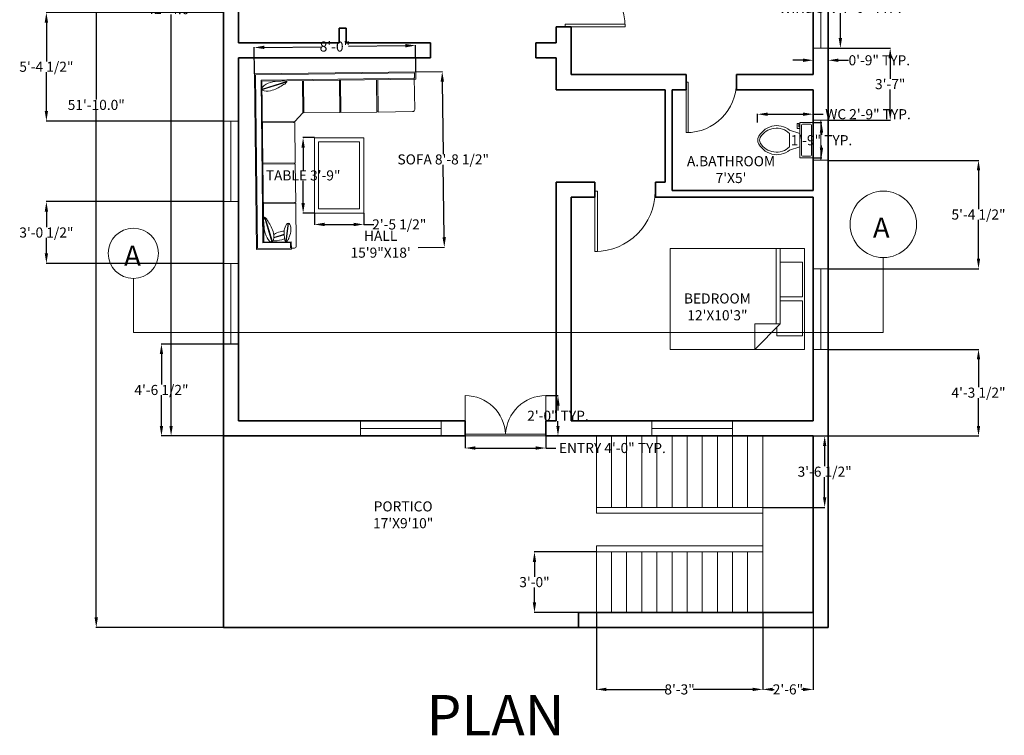
# Model space of a CAD drawing. Units: inches. Extents: x 94 to 277359, y -289541 to 1081.
# Tile 2 of 5: x 94 to 680, y 339 to 765. Entities that reach past the tile are written whole.
import ezdxf

# ---------------------------------------------------------------- set-up
doc = ezdxf.new("R2010")
doc.units = ezdxf.units.IN
doc.header["$MEASUREMENT"] = 0
doc.layers.get('Defpoints').update_dxf_attribs({"color": 255})
for name, color, linetype, lineweight in [('A-ANNO-DIMS', 2, 'Continuous', 18), ('A-ANNO-SYMB', 7, 'Continuous', 18), ('A-ANNO-TEXT', 7, 'Continuous', 30), ('A-AREA-IDEN', 7, 'Continuous', 18), ('A-DOOR', 4, 'Continuous', 18), ('A-FLOR-FIXT', 8, 'Continuous', 18), ('A-WALL', 7, 'Continuous', 35), ('furniture', 163, 'Continuous', 18), ('STAIRCASE', 10, 'Continuous', 18), ('window', 13, 'Continuous', 18)]:
    doc.layers.add(name, color=color, linetype=linetype, lineweight=lineweight)
doc.styles.get("Standard").update_dxf_attribs({"font": 'arial.ttf'})
doc.dimstyles.get("Standard").update_dxf_attribs({"dimtxt": 6, "dimasz": 6, "dimexe": 0.18, "dimexo": 0.0625, "dimgap": 0.09, "dimtad": 0, "dimtih": 1, "dimtoh": 1, "dimdec": 1, "dimzin": 0, "dimdsep": 46, "dimlunit": 3, "dimtxsty": 'Standard', "dimcen": 0.09, "dimadec": 0, "dimazin": 0, "dimtfac": 1, "dimtdec": 1, "dimtofl": 0, "dimtmove": 0, "dimatfit": 3, "dimfxl": 1, "dimtolj": 1, "dimtzin": 0, "dimarcsym": 0})

# ---------------------------------------------------------------- blocks, each defined once
blk = doc.blocks.new('DOOR')
for p, q in [((-94.95, 365.26), (-85.95, 365.26)), ((-94.95, 317.26), (-94.95, 365.26)), ((-90.45, 365.26), (-90.45, 317.26)), ((-85.95, 365.26), (-85.95, 317.26)), ((-85.95, 317.26), (-94.95, 317.26))]:
    blk.add_line(p, q)
blk = doc.blocks.new('V')
for p, q in [((-17.52, 401.92), (-8.52, 401.92)), ((-17.52, 377.92), (-17.52, 401.92)), ((-13.02, 377.92), (-13.02, 401.92)), ((-8.52, 401.92), (-8.52, 377.92)), ((-8.52, 377.92), (-17.52, 377.92))]:
    blk.add_line(p, q)
blk = doc.blocks.new('*D3')
at = {"layer": 'A-ANNO-DIMS', "color": 0, "lineweight": -2, "transparency": 16777216}
for p, q in [((215.5, 1025.45), (139.73, 1025.45)), ((139.91, 1019.45), (139.91, 717.61)), ((139.91, 409.45), (139.91, 711.3)), ((215.5, 403.45), (139.73, 403.45))]:
    blk.add_line(p, q, dxfattribs=at)
at = {"layer": 'A-ANNO-DIMS', "color": 0, "transparency": 16777216}
for points in [[(138.91, 1019.45), (140.91, 1019.45), (139.91, 1025.45)], [(138.91, 409.45), (140.91, 409.45), (139.91, 403.45)]]:
    blk.add_solid(points, dxfattribs=at)
at = {"layer": 'Defpoints', "color": 0, "transparency": 16777216}
for p in [(139.91, 1025.45), (215.56, 1025.45), (215.56, 403.45)]:
    blk.add_point(p, dxfattribs=at)
at = {"layer": 'A-ANNO-DIMS', "color": 0, "transparency": 16777216, "insert": (139.91, 714.45), "char_height": 6, "attachment_point": 5}
blk.add_mtext('\\A1;51\'-10.0"', dxfattribs=at)
blk = doc.blocks.new('*D4')
at = {"layer": 'A-ANNO-DIMS', "color": 0, "lineweight": -2, "transparency": 16777216}
for p, q in [((215.5, 1025.45), (184.27, 1025.45)), ((184.45, 1019.45), (184.45, 774.61)), ((184.45, 523.45), (184.45, 768.3)), ((215.5, 517.45), (184.27, 517.45))]:
    blk.add_line(p, q, dxfattribs=at)
at = {"layer": 'A-ANNO-DIMS', "color": 0, "transparency": 16777216}
for points in [[(183.45, 1019.45), (185.45, 1019.45), (184.45, 1025.45)], [(183.45, 523.45), (185.45, 523.45), (184.45, 517.45)]]:
    blk.add_solid(points, dxfattribs=at)
at = {"layer": 'Defpoints', "color": 0, "transparency": 16777216}
for p in [(215.56, 1025.45), (184.45, 517.45), (215.56, 517.45)]:
    blk.add_point(p, dxfattribs=at)
at = {"layer": 'A-ANNO-DIMS', "color": 0, "transparency": 16777216, "insert": (184.45, 771.45), "char_height": 6, "attachment_point": 5}
blk.add_mtext('\\A1;42\'-4.0"', dxfattribs=at)
blk = doc.blocks.new('sofa')
at = {"layer": 'furniture'}
for p, q in [((350.79, 469.57), (336.2, 465.25)), ((350.63, 469.16), (336.28, 464.99)), ((383.04, 450.77), (383.04, 470.07)), ((406.99, 470.07), (406.99, 450.77)), ((430.99, 455.52), (426.82, 469.87)), ((431.39, 455.35), (427.08, 469.94)), ((338.43, 464.07), (340.23, 457.88)), ((338.72, 464.05), (340.51, 457.89)), ((332.19, 451.9), (332.19, 453.72)), ((336.18, 456.71), (347.07, 455.29)), ((336.2, 456.92), (347.1, 455.5)), ((359.61, 451.29), (358.97, 451.29)), ((359.61, 451.29), (358.97, 451.29)), ((383.04, 451.29), (382.4, 451.29)), ((407.63, 451.29), (406.99, 451.29)), ((358.97, 450.77), (333.46, 450.77)), ((382.39, 450.77), (359.61, 450.77)), ((406.99, 450.77), (383.04, 450.77)), ((413.11, 445.31), (413.11, 445.95)), ((413.11, 423.23), (413.11, 423.87)), ((413.11, 401.16), (413.11, 401.8)), ((413.87, 379.35), (432.81, 379.35))]:
    blk.add_line(p, q, dxfattribs=at)
for points in [[(431.89, 470.07), (431.89, 378.38), (436.22, 378.38), (436.22, 474.39), (331.68, 474.39), (331.68, 453.72), (336.08, 453.73), (336.08, 470.07), (431.89, 470.07)], [(358.97, 450.77), (358.97, 470.07)], [(359.61, 450.77), (359.61, 470.07)], [(382.4, 450.77), (382.4, 470.07)], [(431.89, 445.95), (412.6, 445.95), (407.63, 450.77), (407.63, 470.07)], [(431.89, 423.87), (412.6, 423.87), (412.6, 445.31), (431.89, 445.31)], [(412.6, 401.8), (412.6, 423.23), (431.89, 423.23)], [(431.89, 401.8), (412.6, 401.8)], [(412.6, 380.48), (412.6, 401.16), (431.89, 401.16)]]:
    blk.add_lwpolyline(points, dxfattribs=at)
blk.add_lwpolyline([(335.57, 470.58), (432.4, 470.58), (432.4, 379.24), (435.71, 379.24), (435.71, 473.88), (332.19, 473.88), (332.19, 454.23), (335.57, 454.23)], close=True, dxfattribs=at)
for centre, start, end in [((333.46, 452.05), 186.69307, 269.99993), ((413.87, 380.63), 180.00473, 270.00007)]:
    blk.add_arc(centre, 1.28, start, end, dxfattribs=at)
for points, knots in [([(349.6, 468.13), (349.14, 467.92), (347.75, 466.93), (344.77, 465.38), (341.49, 463.98), (336.52, 463.91), (335.8, 466.54), (340.37, 469.29), (344.16, 469.84), (347.43, 469.89), (349.25, 470.15), (351.26, 469.6), (349.6, 468.13)], [0, 0, 0, 0, 5.78506, 20.019226, 35.456927, 51.784724, 57.97649, 75.904696, 98.086664, 106.437957, 110.953168, 112.080004, 112.080004, 112.080004, 112.080004]), ([(429.95, 456.54), (429.75, 457.01), (428.75, 458.4), (427.21, 461.38), (425.8, 464.66), (425.74, 469.63), (428.37, 470.34), (431.12, 465.78), (431.67, 461.98), (431.72, 458.71), (431.98, 456.9), (431.42, 454.88), (429.95, 456.54)], [0, 0, 0, 0, 5.78506, 20.019226, 35.456927, 51.784724, 57.97649, 75.904696, 98.086664, 106.437957, 110.953168, 112.080004, 112.080004, 112.080004, 112.080004]), ([(337.88, 457.68), (337.9, 457.81), (337.02, 459.85), (336.72, 461.9), (336.65, 464.24), (336.65, 464.58)], [75.416636, 75.416636, 75.416636, 75.416636, 75.904696, 98.086664, 101.64289, 101.64289, 101.64289, 101.64289]), ([(340.47, 464.13), (340.65, 463.77), (341.43, 462.19), (342.13, 460.56), (342.38, 458.63), (342.46, 457.86)], [127.65261, 127.65261, 127.65261, 127.65261, 132.09923, 147.536931, 150.407473, 150.407473, 150.407473, 150.407473]), ([(336.4, 457.25), (336.73, 457.47), (338.07, 457.76), (340.75, 457.94), (343.6, 457.92), (347.27, 456.37), (346.95, 454.21), (342.72, 453.66), (339.77, 454.47), (337.35, 455.49), (336.22, 456.2), (336.14, 456.75), (336.4, 457.25)], [0, 0, 0, 0, 5.78506, 20.019226, 35.456927, 51.784724, 57.97649, 75.904696, 98.086664, 106.437957, 110.953168, 112.080004, 112.080004, 112.080004, 112.080004])]:
    blk.add_open_spline(points, degree=3, knots=knots, dxfattribs=at)
blk = doc.blocks.new('Bed - Queen')
for p, q in [((0, -80.00003), (0, 0)), ((0, 0), (59.99999, 0)), ((59.99999, 0), (59.99999, -80.00003)), ((7.99999, -1.2), (28.79998, -1.2)), ((7.99999, -14.4), (7.99999, -1.2)), ((28.79998, -1.2), (28.79998, -14.4)), ((31.19999, -1.2), (51.99999, -1.2)), ((31.19999, -14.4), (31.19999, -1.2)), ((51.99999, -1.2), (51.99999, -16.4)), ((0, -14.4), (44.8, -14.4)), ((44.8, -16.8), (0, -16.8)), ((59.99999, -29.6), (44.8, -14.4)), ((44.8, -14.4), (44.8, -29.6)), ((51.99999, -16.4), (46.79936, -16.4)), ((44.8, -29.6), (59.99999, -29.6)), ((59.99999, -80.00003), (0, -80.00003))]:
    blk.add_line(p, q)
blk = doc.blocks.new('taBLE')
at = {"layer": 'furniture'}
for points in [[(384.8, 484.44), (429.71, 484.44), (429.71, 455.08), (384.8, 455.08)], [(387.27, 481.97), (427.24, 481.97), (427.24, 457.55), (387.27, 457.55)]]:
    blk.add_lwpolyline(points, close=True, dxfattribs=at)
blk = doc.blocks.new('Toilet - top')
for p, q in [((9.5, -6), (9.5, -2)), ((-10, -8.5), (-8, -8.5)), ((-10, -9.5), (-10, -8.5)), ((-7, -9.5), (-10, -9.5)), ((-8, -8.5), (-8, -8)), ((-7, -8), (-7, -9.5)), ((-4, -8), (-6, -14)), ((4, -8), (6, -14)), ((4, -14), (-4, -14))]:
    blk.add_line(p, q)
blk.add_lwpolyline([(10.5, -8), (10.5, 0), (-10.5, 0), (-10.5, -8)], close=True)
for points in [[(-9.5, -2), (-9.5, -6)], [(8.5, -1), (-8.5, -1)], [(-8.5, -7), (8.5, -7)]]:
    blk.add_lwpolyline(points)
for centre, radius, start, end in [((-8.62, -1.88), 0.884, 81.8699, 188.1301), ((8.62, -1.88), 0.884, 351.8699, 98.1301), ((-8.62, -6.12), 0.884, 171.8699, 278.1301), ((8.62, -6.12), 0.884, 261.8699, 8.1301), ((3.52, -21.58), 12.17, 141.46911, 247.97143), ((4.2, -21.82), 11.33, 136.36773, 238.94682), ((-3.52, -21.58), 12.17, 292.02843, 38.53071), ((-4.2, -21.82), 11.33, 301.05301, 43.63209), ((0, -27.88), 4, 245.73182, 294.26817), ((0, -29), 4, 254.86053, 285.13947)]:
    blk.add_arc(centre, radius, start, end)
blk = doc.blocks.new('MD')
for p, q in [((202.8, 674.18), (202.8, 698.18)), ((250.8, 674.18), (250.8, 698.18)), ((202.8, 675.18), (250.8, 675.18)), ((202.8, 674.18), (250.8, 674.18))]:
    blk.add_line(p, q)
for centre, start, end in [((202.8, 674.18), 2.38802, 90), ((250.8, 674.18), 90, 177.61198)]:
    blk.add_arc(centre, 24, start, end)
blk = doc.blocks.new('*U15')
for p, q in [((0, 0), (0, -6)), ((40, 0), (40, -6))]:
    blk.add_line(p, q)
blk.add_lwpolyline([(0, 0), (0, 40), (1.75, 40), (1.75, 0)], close=True)
blk.add_arc((0, 0), 40, 0, 90)
blk = doc.blocks.new('*D21')
at = {"layer": 'A-ANNO-DIMS', "color": 0, "lineweight": -2, "transparency": 16777216}
for p, q in [((575.63, 796.21), (582.94, 796.21)), ((582.76, 790.21), (582.76, 775.41)), ((582.76, 754.21), (582.76, 769.02)), ((575.63, 748.21), (582.94, 748.21))]:
    blk.add_line(p, q, dxfattribs=at)
at = {"layer": 'A-ANNO-DIMS', "color": 0, "transparency": 16777216}
for points in [[(581.76, 790.21), (583.76, 790.21), (582.76, 796.21)], [(581.76, 754.21), (583.76, 754.21), (582.76, 748.21)]]:
    blk.add_solid(points, dxfattribs=at)
at = {"layer": 'Defpoints', "color": 0, "transparency": 16777216}
for p in [(575.56, 796.21), (582.76, 796.21), (575.56, 748.21)]:
    blk.add_point(p, dxfattribs=at)
at = {"layer": 'A-ANNO-DIMS', "color": 0, "transparency": 16777216, "insert": (582.76, 772.21), "char_height": 6, "attachment_point": 5}
blk.add_mtext('\\A1;WINDOW 4\'-0" TYP.', dxfattribs=at)
blk = doc.blocks.new('*D22')
at = {"layer": 'A-ANNO-DIMS', "color": 0, "lineweight": -2, "transparency": 16777216}
for p, q in [((566.56, 748.15), (566.56, 740.83)), ((575.56, 748.15), (575.56, 740.83)), ((560.56, 741.01), (554.56, 741.01)), ((581.56, 741.01), (587.56, 741.01))]:
    blk.add_line(p, q, dxfattribs=at)
at = {"layer": 'A-ANNO-DIMS', "color": 0, "transparency": 16777216}
for points in [[(560.56, 742.01), (560.56, 740.01), (566.56, 741.01)], [(581.56, 742.01), (581.56, 740.01), (575.56, 741.01)]]:
    blk.add_solid(points, dxfattribs=at)
at = {"layer": 'Defpoints', "color": 0, "transparency": 16777216}
for p in [(566.56, 748.21), (575.56, 748.21), (575.56, 741.01)]:
    blk.add_point(p, dxfattribs=at)
at = {"layer": 'A-ANNO-DIMS', "color": 0, "transparency": 16777216, "insert": (605.94, 741.01), "char_height": 6, "attachment_point": 5}
blk.add_mtext('\\A1;0\'-9" TYP.', dxfattribs=at)
blk = doc.blocks.new('*D29')
at = {"layer": 'A-ANNO-DIMS', "color": 0, "lineweight": -2, "transparency": 16777216}
for p, q in [((533.52, 704.02), (533.52, 709.09)), ((566.56, 704.02), (566.56, 709.09)), ((539.52, 708.91), (560.56, 708.91)), ((566.56, 708.91), (572.56, 708.91))]:
    blk.add_line(p, q, dxfattribs=at)
at = {"layer": 'A-ANNO-DIMS', "color": 0, "transparency": 16777216}
for points in [[(539.52, 709.91), (539.52, 707.91), (533.52, 708.91)], [(560.56, 709.91), (560.56, 707.91), (566.56, 708.91)]]:
    blk.add_solid(points, dxfattribs=at)
at = {"layer": 'Defpoints', "color": 0, "transparency": 16777216}
for p in [(533.52, 703.95), (566.56, 708.91), (566.56, 703.95)]:
    blk.add_point(p, dxfattribs=at)
at = {"layer": 'A-ANNO-DIMS', "color": 0, "transparency": 16777216, "insert": (599.21, 708.91), "char_height": 6, "attachment_point": 5}
blk.add_mtext('\\A1;WC 2\'-9" TYP.', dxfattribs=at)
blk = doc.blocks.new('*D30')
at = {"layer": 'A-ANNO-DIMS', "color": 0, "lineweight": -2, "transparency": 16777216}
for p, q in [((566.63, 703.95), (571.7, 703.95)), ((571.52, 697.95), (571.52, 696.61)), ((571.52, 688.95), (571.52, 690.3)), ((566.63, 682.95), (571.7, 682.95))]:
    blk.add_line(p, q, dxfattribs=at)
at = {"layer": 'A-ANNO-DIMS', "color": 0, "transparency": 16777216}
for points in [[(570.52, 697.95), (572.52, 697.95), (571.52, 703.95)], [(570.52, 688.95), (572.52, 688.95), (571.52, 682.95)]]:
    blk.add_solid(points, dxfattribs=at)
at = {"layer": 'Defpoints', "color": 0, "transparency": 16777216}
for p in [(566.56, 703.95), (566.56, 682.95), (571.52, 682.95)]:
    blk.add_point(p, dxfattribs=at)
at = {"layer": 'A-ANNO-DIMS', "color": 0, "transparency": 16777216, "insert": (571.52, 693.45), "char_height": 6, "attachment_point": 5}
blk.add_mtext('\\A1;1\'-9" TYP.', dxfattribs=at)
blk = doc.blocks.new('*D31')
at = {"layer": 'A-ANNO-DIMS', "color": 0, "lineweight": -2, "transparency": 16777216}
for p, q in [((359.49, 517.39), (359.49, 510.07)), ((407.49, 517.39), (407.49, 510.07)), ((365.49, 510.25), (401.49, 510.25)), ((407.49, 510.25), (413.49, 510.25))]:
    blk.add_line(p, q, dxfattribs=at)
at = {"layer": 'A-ANNO-DIMS', "color": 0, "transparency": 16777216}
for points in [[(365.49, 511.25), (365.49, 509.25), (359.49, 510.25)], [(401.49, 511.25), (401.49, 509.25), (407.49, 510.25)]]:
    blk.add_solid(points, dxfattribs=at)
at = {"layer": 'Defpoints', "color": 0, "transparency": 16777216}
for p in [(359.49, 517.45), (407.49, 517.45), (407.49, 510.25)]:
    blk.add_point(p, dxfattribs=at)
at = {"layer": 'A-ANNO-DIMS', "color": 0, "transparency": 16777216, "insert": (447.08, 510.25), "char_height": 6, "attachment_point": 5}
blk.add_mtext('\\A1;ENTRY 4\'-0" TYP.', dxfattribs=at)
blk = doc.blocks.new('*D32')
at = {"layer": 'A-ANNO-DIMS', "color": 0, "lineweight": -2, "transparency": 16777216}
for p, q in [((407.56, 541.45), (414.87, 541.45)), ((414.69, 535.45), (414.69, 532.61)), ((414.69, 523.45), (414.69, 526.3)), ((407.56, 517.45), (414.87, 517.45))]:
    blk.add_line(p, q, dxfattribs=at)
at = {"layer": 'A-ANNO-DIMS', "color": 0, "transparency": 16777216}
for points in [[(413.69, 535.45), (415.69, 535.45), (414.69, 541.45)], [(413.69, 523.45), (415.69, 523.45), (414.69, 517.45)]]:
    blk.add_solid(points, dxfattribs=at)
at = {"layer": 'Defpoints', "color": 0, "transparency": 16777216}
for p in [(407.49, 541.45), (414.69, 541.45), (407.49, 517.45)]:
    blk.add_point(p, dxfattribs=at)
at = {"layer": 'A-ANNO-DIMS', "color": 0, "transparency": 16777216, "insert": (414.69, 529.45), "char_height": 6, "attachment_point": 5}
blk.add_mtext('\\A1;2\'-0" TYP.', dxfattribs=at)
blk = doc.blocks.new('*D35')
at = {"layer": 'A-ANNO-DIMS', "color": 0, "lineweight": -2, "transparency": 16777216}
for p, q in [((330.18, 734.09), (345.98, 734.28)), ((345.87, 728.27), (346.39, 685.2)), ((346.98, 635.74), (346.46, 678.81)), ((331.43, 629.55), (347.23, 629.74))]:
    blk.add_line(p, q, dxfattribs=at)
at = {"layer": 'A-ANNO-DIMS', "color": 0, "transparency": 16777216}
for points in [[(346.87, 728.29), (344.87, 728.26), (345.8, 734.27)], [(347.98, 635.75), (345.98, 635.72), (347.05, 629.74)]]:
    blk.add_solid(points, dxfattribs=at)
at = {"layer": 'Defpoints', "color": 0, "transparency": 16777216}
for p in [(330.12, 734.09), (345.8, 734.27), (331.37, 629.55)]:
    blk.add_point(p, dxfattribs=at)
at = {"layer": 'A-ANNO-DIMS', "color": 0, "transparency": 16777216, "insert": (346.42, 682.01), "char_height": 6, "attachment_point": 5}
blk.add_mtext('\\A1;SOFA 8\'-8 1/2"', dxfattribs=at)
blk = doc.blocks.new('*D36')
at = {"layer": 'A-ANNO-DIMS', "color": 0, "lineweight": -2, "transparency": 16777216}
for p, q in [((234.11, 733), (233.92, 748.79)), ((239.93, 748.69), (273.86, 749.09)), ((323.93, 749.69), (290, 749.29)), ((330.12, 734.15), (329.93, 749.95))]:
    blk.add_line(p, q, dxfattribs=at)
at = {"layer": 'A-ANNO-DIMS', "color": 0, "transparency": 16777216}
for points in [[(323.92, 750.69), (323.94, 748.69), (329.93, 749.77)], [(239.91, 749.69), (239.94, 747.69), (233.93, 748.61)]]:
    blk.add_solid(points, dxfattribs=at)
at = {"layer": 'Defpoints', "color": 0, "transparency": 16777216}
for p in [(233.93, 748.61), (234.11, 732.93), (330.12, 734.09)]:
    blk.add_point(p, dxfattribs=at)
at = {"layer": 'A-ANNO-DIMS', "color": 0, "transparency": 16777216, "insert": (281.93, 749.19), "char_height": 6, "attachment_point": 5}
blk.add_mtext('\\A1;8\'-0"', dxfattribs=at)
blk = doc.blocks.new('*D37')
at = {"layer": 'A-ANNO-DIMS', "color": 0, "lineweight": -2, "transparency": 16777216}
for p, q in [((269.71, 694.95), (262.85, 694.95)), ((263.03, 688.95), (263.03, 675.65)), ((263.03, 656.04), (263.03, 669.34)), ((269.71, 650.04), (262.85, 650.04))]:
    blk.add_line(p, q, dxfattribs=at)
at = {"layer": 'A-ANNO-DIMS', "color": 0, "transparency": 16777216}
for points in [[(262.03, 688.95), (264.03, 688.95), (263.03, 694.95)], [(262.03, 656.04), (264.03, 656.04), (263.03, 650.04)]]:
    blk.add_solid(points, dxfattribs=at)
at = {"layer": 'Defpoints', "color": 0, "transparency": 16777216}
for p in [(269.77, 694.95), (263.03, 650.04), (269.77, 650.04)]:
    blk.add_point(p, dxfattribs=at)
at = {"layer": 'A-ANNO-DIMS', "color": 0, "transparency": 16777216, "insert": (263.03, 672.49), "char_height": 6, "attachment_point": 5}
blk.add_mtext('\\A1;TABLE 3\'-9"', dxfattribs=at)
blk = doc.blocks.new('*D38')
at = {"layer": 'A-ANNO-DIMS', "color": 0, "lineweight": -2, "transparency": 16777216}
for p, q in [((269.77, 649.97), (269.77, 643.12)), ((299.13, 649.97), (299.13, 643.12)), ((275.77, 643.3), (293.13, 643.3)), ((299.13, 643.3), (305.13, 643.3))]:
    blk.add_line(p, q, dxfattribs=at)
at = {"layer": 'A-ANNO-DIMS', "color": 0, "transparency": 16777216}
for points in [[(275.77, 644.3), (275.77, 642.3), (269.77, 643.3)], [(293.13, 644.3), (293.13, 642.3), (299.13, 643.3)]]:
    blk.add_solid(points, dxfattribs=at)
at = {"layer": 'Defpoints', "color": 0, "transparency": 16777216}
for p in [(269.77, 650.04), (299.13, 650.04), (299.13, 643.3)]:
    blk.add_point(p, dxfattribs=at)
at = {"layer": 'A-ANNO-DIMS', "color": 0, "transparency": 16777216, "insert": (320.24, 643.3), "char_height": 6, "attachment_point": 5}
blk.add_mtext('\\A1;2\'-5 1/2"', dxfattribs=at)
blk = doc.blocks.new('*D45')
at = {"layer": 'A-ANNO-DIMS', "color": 0, "lineweight": -2, "transparency": 16777216}
for p, q in [((437.56, 412.39), (437.56, 366.42)), ((536.56, 412.39), (536.56, 366.42)), ((443.56, 366.6), (478.99, 366.6)), ((530.56, 366.6), (495.13, 366.6))]:
    blk.add_line(p, q, dxfattribs=at)
at = {"layer": 'A-ANNO-DIMS', "color": 0, "transparency": 16777216}
for points in [[(443.56, 367.6), (443.56, 365.6), (437.56, 366.6)], [(530.56, 367.6), (530.56, 365.6), (536.56, 366.6)]]:
    blk.add_solid(points, dxfattribs=at)
at = {"layer": 'Defpoints', "color": 0, "transparency": 16777216}
for p in [(437.56, 412.45), (536.56, 412.45), (536.56, 366.6)]:
    blk.add_point(p, dxfattribs=at)
at = {"layer": 'A-ANNO-DIMS', "color": 0, "transparency": 16777216, "insert": (487.06, 366.6), "char_height": 6, "attachment_point": 5}
blk.add_mtext('\\A1;8\'-3"', dxfattribs=at)
blk = doc.blocks.new('*D46')
at = {"layer": 'A-ANNO-DIMS', "color": 0, "lineweight": -2, "transparency": 16777216}
for p, q in [((536.56, 412.39), (536.56, 366.42)), ((566.56, 412.39), (566.56, 366.42)), ((542.56, 366.6), (543.45, 366.6)), ((560.56, 366.6), (559.68, 366.6))]:
    blk.add_line(p, q, dxfattribs=at)
at = {"layer": 'A-ANNO-DIMS', "color": 0, "transparency": 16777216}
for points in [[(542.56, 367.6), (542.56, 365.6), (536.56, 366.6)], [(560.56, 367.6), (560.56, 365.6), (566.56, 366.6)]]:
    blk.add_solid(points, dxfattribs=at)
at = {"layer": 'Defpoints', "color": 0, "transparency": 16777216}
for p in [(536.56, 412.45), (566.56, 412.45), (566.56, 366.6)]:
    blk.add_point(p, dxfattribs=at)
at = {"layer": 'A-ANNO-DIMS', "color": 0, "transparency": 16777216, "insert": (551.56, 366.6), "char_height": 6, "attachment_point": 5}
blk.add_mtext('\\A1;2\'-6"', dxfattribs=at)
blk = doc.blocks.new('*D47')
at = {"layer": 'A-ANNO-DIMS', "color": 0, "lineweight": -2, "transparency": 16777216}
for p, q in [((437.5, 448.45), (400.53, 448.45)), ((400.71, 442.45), (400.71, 433.61)), ((400.71, 418.45), (400.71, 427.3)), ((437.5, 412.45), (400.53, 412.45))]:
    blk.add_line(p, q, dxfattribs=at)
at = {"layer": 'A-ANNO-DIMS', "color": 0, "transparency": 16777216}
for points in [[(399.71, 442.45), (401.71, 442.45), (400.71, 448.45)], [(399.71, 418.45), (401.71, 418.45), (400.71, 412.45)]]:
    blk.add_solid(points, dxfattribs=at)
at = {"layer": 'Defpoints', "color": 0, "transparency": 16777216}
for p in [(400.71, 448.45), (437.56, 448.45), (437.56, 412.45)]:
    blk.add_point(p, dxfattribs=at)
at = {"layer": 'A-ANNO-DIMS', "color": 0, "transparency": 16777216, "insert": (400.71, 430.45), "char_height": 6, "attachment_point": 5}
blk.add_mtext('\\A1;3\'-0"', dxfattribs=at)
blk = doc.blocks.new('*D48')
at = {"layer": 'A-ANNO-DIMS', "color": 0, "lineweight": -2, "transparency": 16777216}
for p, q in [((536.63, 517.45), (573.59, 517.45)), ((573.41, 511.45), (573.41, 499.36)), ((573.41, 480.89), (573.41, 492.98)), ((536.63, 474.89), (573.59, 474.89))]:
    blk.add_line(p, q, dxfattribs=at)
at = {"layer": 'A-ANNO-DIMS', "color": 0, "transparency": 16777216}
for points in [[(572.41, 511.45), (574.41, 511.45), (573.41, 517.45)], [(572.41, 480.89), (574.41, 480.89), (573.41, 474.89)]]:
    blk.add_solid(points, dxfattribs=at)
at = {"layer": 'Defpoints', "color": 0, "transparency": 16777216}
for p in [(536.56, 517.45), (536.56, 474.89), (573.41, 474.89)]:
    blk.add_point(p, dxfattribs=at)
at = {"layer": 'A-ANNO-DIMS', "color": 0, "transparency": 16777216, "insert": (573.41, 496.17), "char_height": 6, "attachment_point": 5}
blk.add_mtext('\\A1;3\'-6 1/2"', dxfattribs=at)
blk = doc.blocks.new('*D54')
at = {"layer": 'A-ANNO-DIMS', "color": 0, "lineweight": -2, "transparency": 16777216}
for p, q in [((215.5, 572.15), (178.53, 572.15)), ((178.71, 566.15), (178.71, 547.99)), ((178.71, 523.45), (178.71, 541.61)), ((215.5, 517.45), (178.53, 517.45))]:
    blk.add_line(p, q, dxfattribs=at)
at = {"layer": 'A-ANNO-DIMS', "color": 0, "transparency": 16777216}
for points in [[(177.71, 566.15), (179.71, 566.15), (178.71, 572.15)], [(177.71, 523.45), (179.71, 523.45), (178.71, 517.45)]]:
    blk.add_solid(points, dxfattribs=at)
at = {"layer": 'Defpoints', "color": 0, "transparency": 16777216}
for p in [(178.71, 572.15), (215.56, 572.15), (215.56, 517.45)]:
    blk.add_point(p, dxfattribs=at)
at = {"layer": 'A-ANNO-DIMS', "color": 0, "transparency": 16777216, "insert": (178.71, 544.8), "char_height": 6, "attachment_point": 5}
blk.add_mtext('\\A1;4\'-6 1/2"', dxfattribs=at)
blk = doc.blocks.new('*D55')
at = {"layer": 'A-ANNO-DIMS', "color": 0, "lineweight": -2, "transparency": 16777216}
for p, q in [((215.5, 656.86), (110.05, 656.86)), ((110.23, 650.86), (110.23, 641.7)), ((110.23, 626.15), (110.23, 635.31)), ((215.5, 620.15), (110.05, 620.15))]:
    blk.add_line(p, q, dxfattribs=at)
at = {"layer": 'A-ANNO-DIMS', "color": 0, "transparency": 16777216}
for points in [[(109.23, 650.86), (111.23, 650.86), (110.23, 656.86)], [(109.23, 626.15), (111.23, 626.15), (110.23, 620.15)]]:
    blk.add_solid(points, dxfattribs=at)
at = {"layer": 'Defpoints', "color": 0, "transparency": 16777216}
for p in [(110.23, 656.86), (215.56, 656.86), (215.56, 620.15)]:
    blk.add_point(p, dxfattribs=at)
at = {"layer": 'A-ANNO-DIMS', "color": 0, "transparency": 16777216, "insert": (110.23, 638.5), "char_height": 6, "attachment_point": 5}
blk.add_mtext('\\A1;3\'-0 1/2"', dxfattribs=at)
blk = doc.blocks.new('*D56')
at = {"layer": 'A-ANNO-DIMS', "color": 0, "lineweight": -2, "transparency": 16777216}
for p, q in [((215.5, 769.45), (110.05, 769.45)), ((110.23, 763.45), (110.23, 740.35)), ((110.23, 710.86), (110.23, 733.96)), ((215.5, 704.86), (110.05, 704.86))]:
    blk.add_line(p, q, dxfattribs=at)
at = {"layer": 'A-ANNO-DIMS', "color": 0, "transparency": 16777216}
for points in [[(109.23, 763.45), (111.23, 763.45), (110.23, 769.45)], [(109.23, 710.86), (111.23, 710.86), (110.23, 704.86)]]:
    blk.add_solid(points, dxfattribs=at)
at = {"layer": 'Defpoints', "color": 0, "transparency": 16777216}
for p in [(110.23, 769.45), (215.56, 769.45), (215.56, 704.86)]:
    blk.add_point(p, dxfattribs=at)
at = {"layer": 'A-ANNO-DIMS', "color": 0, "transparency": 16777216, "insert": (110.23, 737.16), "char_height": 6, "attachment_point": 5}
blk.add_mtext('\\A1;5\'-4 1/2"', dxfattribs=at)
blk = doc.blocks.new('*D59')
at = {"layer": 'A-ANNO-DIMS', "color": 0, "lineweight": -2, "transparency": 16777216}
for p, q in [((575.63, 568.95), (665.14, 568.95)), ((664.96, 562.95), (664.96, 546.4)), ((664.96, 523.45), (664.96, 540.01)), ((566.63, 517.45), (665.14, 517.45))]:
    blk.add_line(p, q, dxfattribs=at)
at = {"layer": 'A-ANNO-DIMS', "color": 0, "transparency": 16777216}
for points in [[(663.96, 562.95), (665.96, 562.95), (664.96, 568.95)], [(663.96, 523.45), (665.96, 523.45), (664.96, 517.45)]]:
    blk.add_solid(points, dxfattribs=at)
at = {"layer": 'Defpoints', "color": 0, "transparency": 16777216}
for p in [(575.56, 568.95), (566.56, 517.45), (664.96, 517.45)]:
    blk.add_point(p, dxfattribs=at)
at = {"layer": 'A-ANNO-DIMS', "color": 0, "transparency": 16777216, "insert": (664.96, 543.2), "char_height": 6, "attachment_point": 5}
blk.add_mtext('\\A1;4\'-3 1/2"', dxfattribs=at)
blk = doc.blocks.new('*D60')
at = {"layer": 'A-ANNO-DIMS', "color": 0, "lineweight": -2, "transparency": 16777216}
for p, q in [((575.63, 681.45), (665.14, 681.45)), ((664.96, 675.45), (664.96, 652.4)), ((664.96, 622.95), (664.96, 646.01)), ((575.63, 616.95), (665.14, 616.95))]:
    blk.add_line(p, q, dxfattribs=at)
at = {"layer": 'A-ANNO-DIMS', "color": 0, "transparency": 16777216}
for points in [[(663.96, 675.45), (665.96, 675.45), (664.96, 681.45)], [(663.96, 622.95), (665.96, 622.95), (664.96, 616.95)]]:
    blk.add_solid(points, dxfattribs=at)
at = {"layer": 'Defpoints', "color": 0, "transparency": 16777216}
for p in [(575.56, 681.45), (575.56, 616.95), (664.96, 616.95)]:
    blk.add_point(p, dxfattribs=at)
at = {"layer": 'A-ANNO-DIMS', "color": 0, "transparency": 16777216, "insert": (664.96, 649.2), "char_height": 6, "attachment_point": 5}
blk.add_mtext('\\A1;5\'-4 1/2"', dxfattribs=at)
blk = doc.blocks.new('*D61')
at = {"layer": 'A-ANNO-DIMS', "color": 0, "lineweight": -2, "transparency": 16777216}
for p, q in [((575.63, 748.21), (612.59, 748.21)), ((612.41, 742.21), (612.41, 729.99)), ((612.41, 711.45), (612.41, 723.68)), ((575.63, 705.45), (612.59, 705.45))]:
    blk.add_line(p, q, dxfattribs=at)
at = {"layer": 'A-ANNO-DIMS', "color": 0, "transparency": 16777216}
for points in [[(611.41, 742.21), (613.41, 742.21), (612.41, 748.21)], [(611.41, 711.45), (613.41, 711.45), (612.41, 705.45)]]:
    blk.add_solid(points, dxfattribs=at)
at = {"layer": 'Defpoints', "color": 0, "transparency": 16777216}
for p in [(575.56, 748.21), (575.56, 705.45), (612.41, 705.45)]:
    blk.add_point(p, dxfattribs=at)
at = {"layer": 'A-ANNO-DIMS', "color": 0, "transparency": 16777216, "insert": (612.41, 726.83), "char_height": 6, "attachment_point": 5}
blk.add_mtext('\\A1;3\'-7"', dxfattribs=at)

msp = doc.modelspace()

# ---------------------------------------------------------------- linework, layer by layer
at = {"layer": 'A-ANNO-SYMB'}
for p, q in [((608.32, 578.97), (608.32, 623.58)), ((162.01, 611.19), (162.01, 578.97)), ((162.01, 578.97), (608.32, 578.97))]:
    msp.add_line(p, q, dxfattribs=at)
for centre, radius in [((608.32, 643.37), 19.79), ((162.01, 626.12), 14.93)]:
    msp.add_circle(centre, radius, dxfattribs=at)
at = {"layer": 'A-WALL'}
for p, q in [((215.56, 1025.45), (215.56, 403.45)), ((575.56, 403.45), (575.56, 1025.45)), ((566.56, 732.45), (566.56, 900.45)), ((224.56, 811.45), (224.56, 751.45)), ((284.56, 760.07), (288.56, 760.07)), ((284.56, 760.07), (284.56, 751.45)), ((288.56, 760.07), (288.56, 751.45)), ((413.56, 751.45), (413.56, 760.86)), ((413.56, 760.86), (422.56, 760.86)), ((422.56, 732.45), (422.56, 760.86)), ((284.56, 751.45), (224.56, 751.45)), ((338.93, 751.45), (288.56, 751.45)), ((338.93, 742.45), (338.93, 751.45)), ((413.56, 751.45), (401.56, 751.45)), ((401.56, 742.45), (401.56, 751.45)), ((224.56, 742.45), (224.56, 526.45)), ((338.93, 742.45), (224.56, 742.45)), ((413.56, 742.45), (401.56, 742.45)), ((413.56, 723.45), (413.56, 742.45)), ((490.96, 732.45), (422.56, 732.45)), ((490.96, 723.45), (490.96, 732.45)), ((566.56, 732.45), (520.96, 732.45)), ((520.96, 723.45), (520.96, 732.45)), ((478.56, 723.45), (413.56, 723.45)), ((478.56, 668.45), (478.56, 723.45)), ((482.56, 663.45), (482.56, 723.45)), ((490.96, 723.45), (482.56, 723.45)), ((566.56, 723.45), (520.96, 723.45)), ((566.56, 663.45), (566.56, 723.45)), ((413.56, 526.45), (413.56, 668.45)), ((436.68, 668.45), (413.56, 668.45)), ((436.68, 659.45), (436.68, 668.45)), ((478.56, 668.45), (472.68, 668.45)), ((472.68, 659.45), (472.68, 668.45)), ((566.56, 663.45), (482.56, 663.45)), ((422.56, 526.45), (422.56, 659.45)), ((436.68, 659.45), (422.56, 659.45)), ((566.56, 659.45), (472.68, 659.45)), ((566.56, 526.45), (566.56, 659.45)), ((359.49, 526.45), (224.56, 526.45)), ((359.49, 526.45), (359.49, 517.45)), ((413.56, 526.45), (407.49, 526.45)), ((407.49, 526.45), (407.49, 517.45)), ((566.56, 526.45), (422.56, 526.45)), ((359.49, 517.45), (215.56, 517.45)), ((566.56, 517.45), (407.49, 517.45)), ((566.56, 412.45), (566.56, 517.45)), ((426.95, 412.45), (566.56, 412.45)), ((426.95, 412.45), (426.95, 403.45)), ((215.56, 403.45), (575.56, 403.45))]:
    msp.add_line(p, q, dxfattribs=at)
at = {"layer": 'STAIRCASE'}
for p, q in [((437.56, 471.43), (437.56, 517.45)), ((446.56, 474.89), (446.56, 517.45)), ((455.56, 474.89), (455.56, 517.45)), ((464.56, 474.89), (464.56, 517.45)), ((473.56, 474.89), (473.56, 517.45)), ((482.56, 474.89), (482.56, 517.45)), ((491.56, 474.89), (491.56, 517.45)), ((500.56, 474.89), (500.56, 517.45)), ((509.56, 474.89), (509.56, 517.45)), ((518.56, 474.89), (518.56, 517.45)), ((527.56, 474.89), (527.56, 517.45)), ((536.56, 412.45), (536.56, 517.45)), ((536.56, 474.89), (437.56, 474.89)), ((437.56, 471.43), (536.56, 471.43)), ((536.56, 452.13), (437.56, 452.13)), ((437.56, 412.45), (437.56, 452.13)), ((536.56, 448.45), (536.56, 452.13)), ((437.56, 448.45), (536.56, 448.45)), ((446.56, 412.45), (446.56, 448.45)), ((455.56, 412.45), (455.56, 448.45)), ((464.56, 412.45), (464.56, 448.45)), ((473.56, 412.45), (473.56, 448.45)), ((482.56, 412.45), (482.56, 448.45)), ((491.56, 412.45), (491.56, 448.45)), ((500.56, 412.45), (500.56, 448.45)), ((509.56, 412.45), (509.56, 448.45)), ((518.56, 412.45), (518.56, 448.45)), ((527.56, 412.45), (527.56, 448.45))]:
    msp.add_line(p, q, dxfattribs=at)
at = {"layer": 'window'}
for p, q in [((566.56, 748.21), (575.56, 748.21)), ((224.56, 704.86), (224.56, 704.86)), ((224.56, 581.71), (224.56, 581.71)), ((224.56, 572.15), (215.56, 572.15))]:
    msp.add_line(p, q, dxfattribs=at)

# ---------------------------------------------------------------- block references
at = {"layer": 'A-DOOR'}
for p, xscale, yscale, zscale, rotation in [((418.92, 760.86), -0.8921197571226785, 0.8921197571226785, 0.8921197571226785, 270), ((490.96, 727.95), -0.7503958823192237, 0.7503958823192237, 0.7503958823192237, 180), ((436.68, 663.08), -0.895864590374933, 0.895864590374933, 0.895864590374933, 180)]:
    msp.add_blockref('*U15', p, dxfattribs=dict(at, xscale=xscale, yscale=yscale, zscale=zscale, rotation=rotation))
msp.add_blockref('MD', (156.7, -156.72), dxfattribs=at)
at = {"layer": 'A-FLOR-FIXT', "rotation": 270}
msp.add_blockref('Toilet - top', (566.56, 693.45), dxfattribs=at)
at = {"layer": 'furniture'}
for name, p, rotation in [('sofa', (713.71, 302.44), 90.68742412687722), ('taBLE', (-185.31, 1079.74), 270), ('Bed - Queen', (561.37, 628.95), 270)]:
    msp.add_blockref(name, p, dxfattribs=dict(at, rotation=rotation))
at = {"layer": 'window'}
for name, p in [('DOOR', (661.51, 430.96)), ('DOOR', (310.51, 339.6)), ('V', (584.08, 303.54)), ('DOOR', (310.51, 254.9)), ('DOOR', (661.51, 251.7))]:
    msp.add_blockref(name, p, dxfattribs=at)
at = {"layer": 'window', "rotation": 90}
for p in [(662.51, 612.41), (835.82, 612.41)]:
    msp.add_blockref('DOOR', p, dxfattribs=at)

# ---------------------------------------------------------------- texts
at = {"layer": 'A-ANNO-SYMB', "char_height": 12, "attachment_point": 1}
for insert in [(602.14, 647.39), (156.5, 630.74)]:
    msp.add_mtext_dynamic_manual_height_columns('A', width=7.2178, gutter_width=1, heights=[0], dxfattribs=dict(at, insert=insert))
at = {"layer": 'A-ANNO-TEXT', "insert": (377.53, 363.28), "char_height": 24, "attachment_point": 2}
msp.add_mtext_dynamic_manual_height_columns('PLAN ', width=54.0436, gutter_width=1, heights=[0], dxfattribs=at)
at = {"layer": 'A-AREA-IDEN', "char_height": 6, "attachment_point": 2}
for s, insert in [("A.BATHROOM\\P7'X5'", (517.68, 683.94)), ('HALL\\P15\'9"X18\'', (309.16, 639.51)), ('BEDROOM\\P12\'X10\'3"', (509.59, 602.25)), ('PORTICO\\P17\'X9\'10"', (322.56, 478.51))]:
    msp.add_mtext_dynamic_manual_height_columns(s, width=54.0436, gutter_width=1, heights=[0], dxfattribs=dict(at, insert=insert))

# ---------------------------------------------------------------- dimensions: what is measured, and where the dimension line sits
at = {"layer": 'A-ANNO-DIMS'}
for base, p1, p2, angle, override, picture, middle in [((139.91, 1025.45), (215.56, 403.45), (215.56, 1025.45), 90, {"dimclrd": 0, "dimclre": 0, "dimclrt": 0}, '*D3', (139.91, 714.45)), ((184.45, 517.45), (215.56, 1025.45), (215.56, 517.45), 90, {"dimclrd": 0, "dimclre": 0, "dimclrt": 0}, '*D4', (184.45, 771.45)), ((110.23, 769.45), (215.56, 704.86), (215.56, 769.45), 90, {"dimdec": 1, "dimlfac": 1, "dimrnd": 0, "dimzin": 1, "dimdsep": 46, "dimlunit": 4, "dimfrac": 2}, '*D56', (110.23, 737.16)), ((233.93, 748.61), (330.12, 734.09), (234.11, 732.93), 180.68742, {"dimdec": 1, "dimlfac": 1, "dimrnd": 0, "dimzin": 1, "dimdsep": 46, "dimlunit": 4, "dimfrac": 2}, '*D36', (281.93, 749.19)), ((612.41, 705.45), (575.56, 748.21), (575.56, 705.45), 270, {"dimdec": 1, "dimlfac": 1, "dimrnd": 0, "dimzin": 1, "dimdsep": 46, "dimlunit": 4, "dimfrac": 2}, '*D61', (612.41, 726.83)), ((664.96, 616.95), (575.56, 681.45), (575.56, 616.95), 90, {"dimdec": 1, "dimlfac": 1, "dimrnd": 0, "dimzin": 1, "dimdsep": 46, "dimlunit": 4, "dimfrac": 2}, '*D60', (664.96, 649.2)), ((110.23, 656.86), (215.56, 620.15), (215.56, 656.86), 90, {"dimdec": 1, "dimlfac": 1, "dimrnd": 0, "dimzin": 1, "dimdsep": 46, "dimlunit": 4, "dimfrac": 2}, '*D55', (110.23, 638.5)), ((178.71, 572.15), (215.56, 517.45), (215.56, 572.15), 90, {"dimdec": 1, "dimlfac": 1, "dimrnd": 0, "dimzin": 1, "dimdsep": 46, "dimlunit": 4, "dimfrac": 2}, '*D54', (178.71, 544.8)), ((664.96, 517.45), (575.56, 568.95), (566.56, 517.45), 90, {"dimdec": 1, "dimlfac": 1, "dimrnd": 0, "dimzin": 1, "dimdsep": 46, "dimlunit": 4, "dimfrac": 2}, '*D59', (664.96, 543.2)), ((573.41, 474.89), (536.56, 517.45), (536.56, 474.89), 270, {"dimdec": 1, "dimlfac": 1, "dimrnd": 0, "dimzin": 1, "dimdsep": 46, "dimlunit": 4, "dimfrac": 2}, '*D48', (573.41, 496.17)), ((400.71, 448.45), (437.56, 412.45), (437.56, 448.45), 90, {"dimdec": 1, "dimlfac": 1, "dimrnd": 0, "dimzin": 1, "dimdsep": 46, "dimlunit": 4, "dimfrac": 2}, '*D47', (400.71, 430.45))]:
    dim = msp.add_linear_dim(base=base, p1=p1, p2=p2, angle=angle, dimstyle='Standard', override=override, dxfattribs=at)
    dim.commit()
    dim.dimension.update_dxf_attribs({"geometry": picture, "text_midpoint": middle})
for base, p1, p2, angle, text, picture, middle in [((582.76, 796.21), (575.56, 748.21), (575.56, 796.21), 90, 'WINDOW <> TYP.', '*D21', (582.76, 772.21)), ((345.8, 734.27), (331.37, 629.55), (330.12, 734.09), 90.68742, 'SOFA <>', '*D35', (346.42, 682.01)), ((571.52, 682.95), (566.56, 703.95), (566.56, 682.95), 270, '<> TYP.', '*D30', (571.52, 693.45)), ((263.03, 650.04), (269.77, 694.95), (269.77, 650.04), 270, 'TABLE <>', '*D37', (263.03, 672.49)), ((414.69, 541.45), (407.49, 517.45), (407.49, 541.45), 90, '<> TYP.', '*D32', (414.69, 529.45))]:
    dim = msp.add_linear_dim(base=base, p1=p1, p2=p2, angle=angle, text=text, dimstyle='Standard', override={"dimdec": 1, "dimlfac": 1, "dimrnd": 0, "dimzin": 1, "dimdsep": 46, "dimlunit": 4, "dimfrac": 2}, dxfattribs=at)
    dim.commit()
    dim.dimension.update_dxf_attribs({"geometry": picture, "text_midpoint": middle})
for base, p1, p2, text, picture, middle in [((575.56, 741.01), (566.56, 748.21), (575.56, 748.21), '<> TYP.', '*D22', (605.94, 741.01)), ((566.56, 708.91), (533.52, 703.95), (566.56, 703.95), 'WC <> TYP.', '*D29', (599.21, 708.91)), ((407.49, 510.25), (359.49, 517.45), (407.49, 517.45), 'ENTRY <> TYP.', '*D31', (447.08, 510.25))]:
    dim = msp.add_linear_dim(base=base, p1=p1, p2=p2, text=text, dimstyle='Standard', override={"dimdec": 1, "dimlfac": 1, "dimrnd": 0, "dimzin": 1, "dimdsep": 46, "dimlunit": 4, "dimfrac": 2}, dxfattribs=at)
    dim.commit()
    dim.dimension.update_dxf_attribs({"geometry": picture, "text_midpoint": middle})
for base, p1, p2, picture, middle in [((299.13, 643.3), (269.77, 650.04), (299.13, 650.04), '*D38', (320.24, 643.3)), ((536.56, 366.6), (437.56, 412.45), (536.56, 412.45), '*D45', (487.06, 366.6)), ((566.56, 366.6), (536.56, 412.45), (566.56, 412.45), '*D46', (551.56, 366.6))]:
    dim = msp.add_linear_dim(base=base, p1=p1, p2=p2, dimstyle='Standard', override={"dimdec": 1, "dimlfac": 1, "dimrnd": 0, "dimzin": 1, "dimdsep": 46, "dimlunit": 4, "dimfrac": 2}, dxfattribs=at)
    dim.commit()
    dim.dimension.update_dxf_attribs({"geometry": picture, "text_midpoint": middle})

doc.saveas('drawing.dxf')
